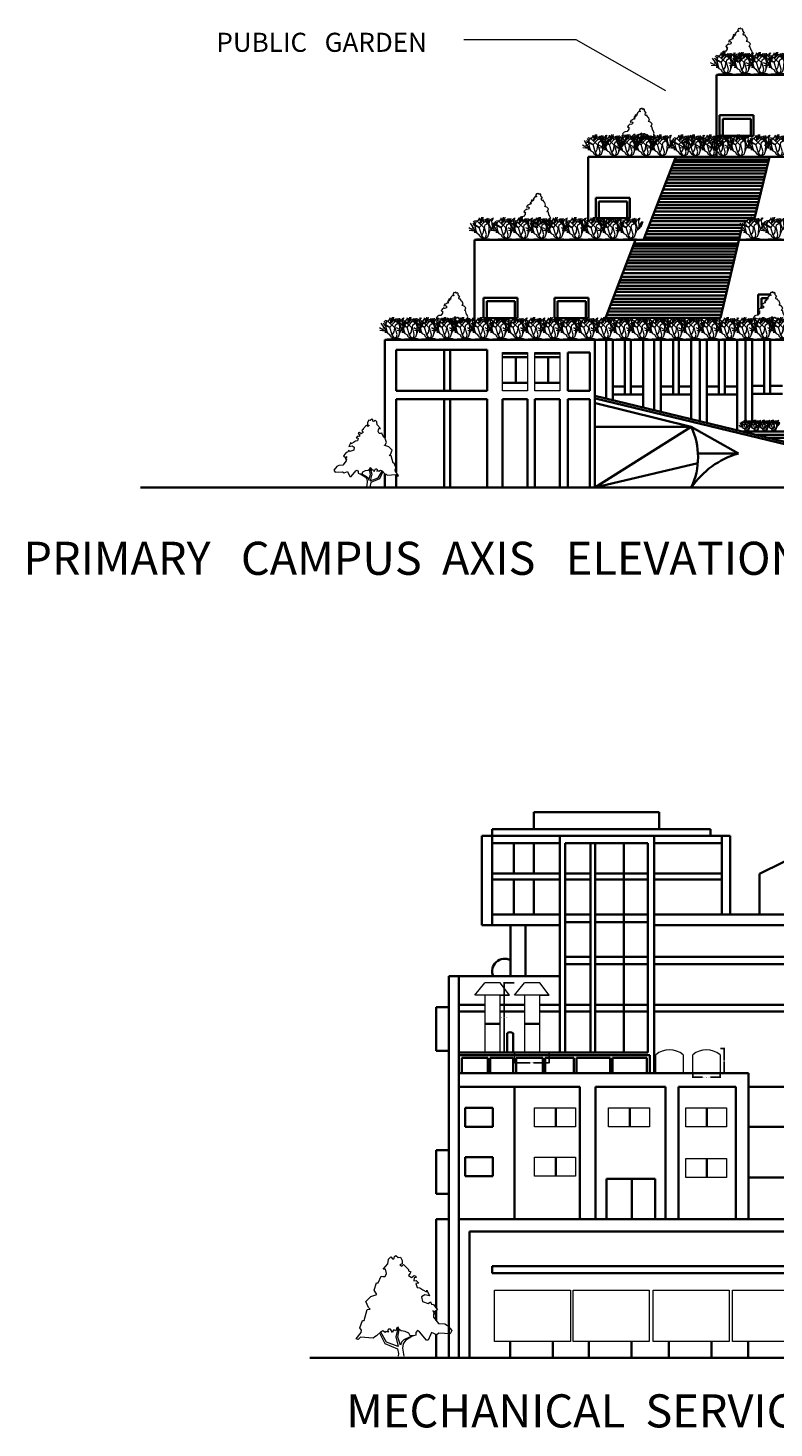
# Model space of a CAD drawing. Units: inches. Extents: x -362 to 223, y -437 to 70.
# Tile 1 of 5: x -362 to -124, y -437 to 8. Entities that reach past the tile are written whole.
import ezdxf

# ---------------------------------------------------------------- set-up
doc = ezdxf.new("R2010")
doc.units = ezdxf.units.IN
doc.header["$MEASUREMENT"] = 0
for name, color, linetype, lineweight in [('A-ANNO-DIMS', 2, 'Continuous', 18), ('A-ANNO-SYMB', 7, 'Continuous', 18), ('A-ANNO-TEXT', 7, 'Continuous', 25), ('A-ELEV', 7, 'Continuous', 35), ('A-EQPM', 8, 'Continuous', 18), ('A-GLAZ', 4, 'Continuous', 18), ('L-PLNT', 3, 'Continuous', 13)]:
    doc.layers.add(name, color=color, linetype=linetype, lineweight=lineweight)
doc.styles.get("Standard").update_dxf_attribs({"font": 'arial.ttf'})
doc.dimstyles.get("Standard").update_dxf_attribs({"dimtxt": 0.18, "dimasz": 0.18, "dimexe": 0.18, "dimexo": 0.0625, "dimgap": 0.09, "dimtad": 0, "dimtih": 1, "dimtoh": 1, "dimdec": 4, "dimzin": 0, "dimdsep": 46, "dimtxsty": 'Standard', "dimcen": 0.09, "dimadec": 0, "dimazin": 0, "dimtfac": 1, "dimtdec": 4, "dimtofl": 0, "dimtmove": 0, "dimatfit": 3, "dimfxl": 1, "dimtolj": 1, "dimtzin": 0, "dimarcsym": 0})

# ---------------------------------------------------------------- blocks, each defined once
blk = doc.blocks.new('*U2')
for points in [[(22.0124, 137.721), (18.5475, 141.5624), (15.5282, 138.2446), (13.8028, 139.3505), (13.3714, 142.1153), (11.2148, 143.2214), (8.1954, 140.4564), (4.7447, 141.0094), (2.1567, 136.0326), (2.1567, 131.6088), (5.6074, 129.9499), (3.0193, 128.2909), (0.4313, 130.5029), (-6.9015, 123.3141), (-6.9015, 121.6552), (-9.9208, 119.9963), (-9.0581, 118.3373), (-6.9015, 115.0195), (-10.7835, 112.2546), (-14.6656, 115.0195), (-16.8222, 114.4665), (-17.6849, 112.2546), (-14.6656, 111.7016), (-14.2342, 107.2778), (-17.6065, 107.8307), (-21.5669, 103.9599), (-17.2536, 103.4069), (-18.9789, 97.8771), (-22.8609, 97.3241), (-27.1743, 94.5593), (-32.3504, 91.7944), (-32.7817, 94.0063), (-36.6638, 85.7116), (-29.7624, 87.3705), (-25.449, 84.6056), (-26.743, 77.9699), (-34.507, 75.205), (-37.9578, 77.4169), (-39.2518, 74.099), (-42.2711, 73.5461), (-44.8592, 70.2282), (-47.8786, 66.3574), (-43.9965, 63.0395), (-41.4085, 64.6985), (-44.3346, 59.8898), (-42.2089, 60.1377), (-42.5159, 55.7849), (-49.6039, 46.4502), (-58.2307, 45.8972), (-62.1127, 43.6853), (-68.5828, 36.4966), (-65.9947, 32.0727), (-50.0352, 32.6257), (-47.0159, 30.4138), (-39.6831, 33.7317), (-34.507, 22.6721), (-32.3504, 22.6721), (-22.4296, 34.8376), (-19.4102, 36.4966), (-17.2536, 33.7317), (-17.2536, 29.8608), (-13.8028, 28.7549), (-9.0581, 28.7549), (-7.3328, 32.6257), (-1.7254, 35.3906), (3.8821, 35.9436), (6.4701, 38.1555), (6.9014, 38.7085), (8.1954, 41.4734), (9.9208, 40.3674), (11.2148, 35.9436), (14.2341, 37.6025), (15.0968, 36.4966), (15.9595, 33.7317), (18.9789, 38.7085), (21.9982, 38.7085), (23.2922, 36.4966), (21.9982, 34.2847), (25.4489, 35.3906), (26.743, 33.7317), (29.7623, 35.9436), (32.7817, 34.8376), (38.8204, 28.7549), (41.4084, 27.6489), (43.5651, 25.437), (61.6813, 27.0959), (65.132, 23.7781), (67.7201, 24.884), (60.8186, 33.7317), (60.3873, 37.0495), (62.544, 40.3674), (58.662, 50.874), (56.5053, 50.874), (52.1919, 66.3574), (47.8785, 66.9103), (50.4665, 69.1222), (53.9172, 77.9699), (47.0158, 85.1586), (38.3891, 87.9235), (42.2711, 94.0063)], [(42.2711, 94.0063), (38.8204, 104.5129), (36.6637, 104.5129), (32.3503, 113.9135), (29.7623, 113.3605), (26.743, 113.3605), (24.5862, 117.7844), (25.8802, 123.8671), (29.331, 123.8671), (22.8609, 131.6088), (21.9982, 137.6916)], [(8.1954, 40.3674), (11.2148, 27.6489), (8.1954, 13.8245), (24.5862, 19.9072), (32.7817, 34.2847)], [(-12.9401, 28.7549), (-2.588, 22.1191), (0.8626, 17.6953), (1.7253, 11.6125), (0, 0)], [(-9.9208, 28.2019), (0, 23.2251), (3.4507, 19.9072), (4.7447, 15.4834), (8.6267, 27.0959), (6.4701, 37.6025)], [(34.5071, 33.1787), (27.1743, 18.2483), (9.0581, 10.5066), (7.7641, 3.8708), (8.1954, 0)]]:
    blk.add_lwpolyline(points)
blk = doc.blocks.new('*U4')
for p, q in [((-18.24, 11.04), (-21.755, 16.655)), ((-12.96, 12.48), (-19.68, 16.32)), ((-13.92, 12.48), (-19.2, 14.88)), ((-16.8, 16.32), (-18.72, 18.72)), ((-14.88, 18.24), (-17.76, 19.2)), ((-16.8, 16.32), (-15.36, 19.68)), ((-16.8, 12.48), (-16.8, 16.32)), ((-14.88, 18.24), (-12.96, 20.64)), ((-8.16, 12), (-14.88, 18.24)), ((-13.325, 16.724), (-11.433, 18.289)), ((-12.96, 12.48), (-8.16, 17.76)), ((-12.471, 19.775), (-12.898, 22.044)), ((-11.677, 19.071), (-12.471, 19.775)), ((-11.28, 19.619), (-12.104, 21.184)), ((-12.043, 15.628), (-11.921, 18.836)), ((-11.982, 16.802), (-10.579, 18.054)), ((-11.921, 18.836), (-10.64, 20.401)), ((-11.433, 18.289), (-10.457, 22.749)), ((-10.579, 18.054), (-9.846, 19.697)), ((-8.16, 17.76), (-10.56, 21.6)), ((-9.48, 19.775), (-8.992, 22.592)), ((-7.2, 19.68), (-8.64, 20.16)), ((-8.16, 17.76), (-5.28, 19.2)), ((-7.68, 12.48), (-7.2, 14.88)), ((-7.2, 19.68), (-6.24, 21.12)), ((-4.8, 16.32), (-7.2, 19.68)), ((-7.2, 14.88), (-3.84, 16.8)), ((-5.086, 17.741), (-5.513, 21.34)), ((-5.28, 19.2), (-3.84, 21.6)), ((-3.377, 15.315), (-5.086, 17.819)), ((-2.88, 12.96), (-4.32, 19.68)), ((-3.84, 16.8), (-0.96, 20.64)), ((-3.377, 18.602), (-2.888, 21.575)), ((-2.766, 16.802), (-3.377, 18.602)), ((-2.88, 15.84), (-2.4, 20.16)), ((-0.96, 10.56), (-2.88, 15.84)), ((-0.508, 21.888), (-0.081, 20.558)), ((-0.203, 19.149), (0.102, 21.34)), ((0.346, 13.203), (-0.203, 19.149)), ((-0.142, 19.384), (0.59, 20.401)), ((-0.02, 20.01), (0.896, 21.105)), ((0.041, 20.714), (1.384, 22.044)), ((0.102, 21.34), (0.835, 21.888)), ((0.346, 13.203), (1.323, 16.254)), ((0.96, 12), (1.44, 15.36)), ((0.96, 12), (2.88, 14.88)), ((1.323, 16.254), (3.642, 18.289)), ((1.44, 15.36), (2.88, 17.28)), ((1.92, 13.44), (2.4, 15.36)), ((2.4, 15.36), (3.36, 16.32)), ((-17.76, 8.64), (-23.663, 11.961)), ((-17.76, 8.64), (-23.128, 9.222)), ((-18.24, 11.04), (-20.16, 11.52)), ((-15.84, 8.16), (-18.24, 11.04)), ((-16.32, 7.2), (-18.24, 7.2)), ((-16.8, 12.48), (-17.76, 12.96)), ((-14.88, 5.76), (-17.76, 8.64)), ((-15.84, 0.48), (-17.76, 0)), ((-15.84, 8.16), (-16.8, 12.48)), ((-14.88, 5.76), (-15.84, 8.16)), ((-13.44, 0.48), (-15.84, 0.48)), ((-12.96, 4.8), (-14.88, 5.76)), ((-12.96, 12.48), (-13.92, 12.48)), ((-9.6, 0.96), (-13.44, 0.48)), ((-10.56, 4.32), (-12.96, 12.48)), ((-11.52, 2.4), (-12.96, 4.8)), ((-9.6, 0.96), (-12.96, 0)), ((-8.64, 0.96), (-11.52, 2.4)), ((-10.56, 4.32), (-8.64, 7.68)), ((-8.64, 1.92), (-10.56, 4.32)), ((-9.6, 0.96), (-7.68, 0.96)), ((-8.64, 7.68), (-8.16, 12)), ((-8.64, 0.96), (-4.32, 2.88)), ((-8.64, 0.96), (-6.24, 2.88)), ((-8.64, 0.96), (-8.64, 1.92)), ((-8.64, 0.96), (-2.88, 0.96)), ((-6.72, 8.64), (-7.68, 12.48)), ((-7.68, 0.96), (-6.24, 0.48)), ((-5.76, 5.28), (-6.72, 8.64)), ((-6.24, 2.88), (-5.76, 5.28)), ((-6.24, 0.48), (-3.36, 0)), ((-4.32, 2.88), (-1.92, 9.6)), ((-3.36, 5.28), (-2.88, 12.96)), ((-2.88, 0.96), (0, 0)), ((-1.92, 9.6), (0.96, 12)), ((-0.48, 10.8), (0.346, 13.203))]:
    blk.add_line(p, q)
blk = doc.blocks.new('WIN-PANEL-A')
for p, q in [((0, 12.16), (7.9, 12.16)), ((0, 0), (0, 12.16)), ((7.9, 12.16), (7.9, 0)), ((7.9, 0), (0, 0))]:
    blk.add_line(p, q)
blk = doc.blocks.new('WIN-STOREFRONT')
for p, q in [((24.23, 16.39), (0, 16.39)), ((0, 16.39), (0, 0)), ((24.23, 0), (24.23, 16.39)), ((0, 0), (6.79, 0)), ((6.79, 0), (24.23, 0))]:
    blk.add_line(p, q)
blk = doc.blocks.new('ROOF-VENT')
for p, q in [((0, 18.24), (2.99, 22.1)), ((2.99, 18.24), (0, 18.24)), ((0, 18.24), (11.03, 18.24)), ((2.99, 22.1), (7.83, 22.1)), ((2.99, 0), (2.99, 18.24)), ((2.99, 18.24), (7.83, 18.24)), ((11.03, 18.24), (7.83, 22.1)), ((7.83, 18.24), (7.83, 0))]:
    blk.add_line(p, q)
blk = doc.blocks.new('WIN-C')
for p, q in [((13.02, 6.07), (0, 6.07)), ((0, 6.07), (0, 5.53)), ((0, 5.53), (0, 0)), ((13.02, 0), (13.02, 6.07)), ((0, 0), (13.02, 0))]:
    blk.add_line(p, q)
blk = doc.blocks.new('WIN-D')
for p, q in [((13.02, 6.07), (0, 6.07)), ((0, 6.07), (0, 5.53)), ((0, 5.53), (0, 0)), ((13.02, 6.07), (11.9, 6.07)), ((13.02, 0), (13.02, 6.07)), ((0, 0), (13.02, 0)), ((11.9, 0), (13.02, 0))]:
    blk.add_line(p, q)
blk = doc.blocks.new('ROOF-DOME')
for p, q in [((0, 0), (0, 5.87)), ((8.74, 5.87), (8.74, 0))]:
    blk.add_line(p, q)
blk.add_arc((4.37, 0.37), 7.03, 51.5309, 128.4691)
blk = doc.blocks.new('*D27')
at = {"layer": 'A-ANNO-DIMS', "color": 0, "lineweight": -2, "transparency": 16777216}
for p, q in [((-207, -295.53), (-210.43, -295.53)), ((-210.25, -295.71), (-210.25, -306.39)), ((-210.25, -317.45), (-210.25, -306.76)), ((-207, -317.63), (-210.43, -317.63))]:
    blk.add_line(p, q, dxfattribs=at)
at = {"layer": 'A-ANNO-DIMS', "color": 0, "transparency": 16777216}
for points in [[(-210.28, -295.71), (-210.22, -295.71), (-210.25, -295.53)], [(-210.28, -317.45), (-210.22, -317.45), (-210.25, -317.63)]]:
    blk.add_solid(points, dxfattribs=at)
at = {"layer": 'Defpoints', "color": 0, "transparency": 16777216}
for p in [(-210.25, -295.53), (-206.94, -295.53), (-206.94, -317.63)]:
    blk.add_point(p, dxfattribs=at)
at = {"layer": 'A-ANNO-DIMS', "color": 0, "transparency": 16777216, "insert": (-210.25, -306.58), "char_height": 0.18, "attachment_point": 5}
blk.add_mtext('\\A1;ROOF VENT 22 TYP.', dxfattribs=at)
blk = doc.blocks.new('*D28')
at = {"layer": 'A-ANNO-DIMS', "color": 0, "lineweight": -2, "transparency": 16777216}
for p, q in [((-206.94, -317.69), (-206.94, -321.12)), ((-195.91, -317.69), (-195.91, -321.12)), ((-206.76, -320.94), (-201.94, -320.94)), ((-196.09, -320.94), (-200.9, -320.94))]:
    blk.add_line(p, q, dxfattribs=at)
at = {"layer": 'A-ANNO-DIMS', "color": 0, "transparency": 16777216}
for points in [[(-206.76, -320.91), (-206.76, -320.97), (-206.94, -320.94)], [(-196.09, -320.91), (-196.09, -320.97), (-195.91, -320.94)]]:
    blk.add_solid(points, dxfattribs=at)
at = {"layer": 'Defpoints', "color": 0, "transparency": 16777216}
for p in [(-206.94, -317.63), (-195.91, -317.63), (-206.94, -320.94)]:
    blk.add_point(p, dxfattribs=at)
at = {"layer": 'A-ANNO-DIMS', "color": 0, "transparency": 16777216, "insert": (-201.42, -320.94), "char_height": 0.18, "attachment_point": 5}
blk.add_mtext('\\A1;11 TYP.', dxfattribs=at)
blk = doc.blocks.new('*D31')
at = {"layer": 'A-ANNO-DIMS', "color": 0, "lineweight": -2, "transparency": 16777216}
for p, q in [((-150.17, -324.32), (-150.17, -325.75)), ((-141.42, -324.32), (-141.42, -325.75)), ((-149.99, -325.57), (-147.06, -325.57)), ((-141.6, -325.57), (-144.53, -325.57))]:
    blk.add_line(p, q, dxfattribs=at)
at = {"layer": 'A-ANNO-DIMS', "color": 0, "transparency": 16777216}
for points in [[(-149.99, -325.54), (-149.99, -325.6), (-150.17, -325.57)], [(-141.6, -325.54), (-141.6, -325.6), (-141.42, -325.57)]]:
    blk.add_solid(points, dxfattribs=at)
at = {"layer": 'Defpoints', "color": 0, "transparency": 16777216}
for p in [(-150.17, -324.26), (-141.42, -324.26), (-141.42, -325.57)]:
    blk.add_point(p, dxfattribs=at)
at = {"layer": 'A-ANNO-DIMS', "color": 0, "transparency": 16777216, "insert": (-145.8, -325.57), "char_height": 0.18, "attachment_point": 5}
blk.add_mtext('\\A1;ROOF DOME 9 TYP.', dxfattribs=at)
blk = doc.blocks.new('*D32')
at = {"layer": 'A-ANNO-DIMS', "color": 0, "lineweight": -2, "transparency": 16777216}
for p, q in [((-141.36, -316.35), (-139.93, -316.35)), ((-140.11, -316.53), (-140.11, -320.12)), ((-140.11, -324.08), (-140.11, -320.49)), ((-141.36, -324.26), (-139.93, -324.26))]:
    blk.add_line(p, q, dxfattribs=at)
at = {"layer": 'A-ANNO-DIMS', "color": 0, "transparency": 16777216}
for points in [[(-140.14, -316.53), (-140.08, -316.53), (-140.11, -316.35)], [(-140.14, -324.08), (-140.08, -324.08), (-140.11, -324.26)]]:
    blk.add_solid(points, dxfattribs=at)
at = {"layer": 'Defpoints', "color": 0, "transparency": 16777216}
for p in [(-141.42, -316.35), (-140.11, -316.35), (-141.42, -324.26)]:
    blk.add_point(p, dxfattribs=at)
at = {"layer": 'A-ANNO-DIMS', "color": 0, "transparency": 16777216, "insert": (-140.11, -320.3), "char_height": 0.18, "attachment_point": 5}
blk.add_mtext('\\A1;8 TYP.', dxfattribs=at)

msp = doc.modelspace()

# ---------------------------------------------------------------- linework, layer by layer
at = {"layer": 'A-ANNO-SYMB'}
for p, q in [((-187.3, 4.66), (-223.08, 4.66)), ((-158.77, -11.54), (-187.3, 4.66))]:
    msp.add_line(p, q, dxfattribs=at)
at = {"layer": 'A-ELEV'}
for p, q in [((-62.22, -6.5), (-142.63, -6.5)), ((-142.63, -6.5), (-142.63, -25.83)), ((-141.63, -25.83), (-141.63, -19.35)), ((-141.63, -19.35), (-130.81, -19.35)), ((-140.6, -20.44), (-131.66, -20.44)), ((-140.6, -25.83), (-140.6, -20.44)), ((-131.66, -25.83), (-131.66, -20.44)), ((-130.81, -19.35), (-130.81, -25.83)), ((-142.63, -25.83), (-142.63, -32.58)), ((-141.63, -25.83), (-130.81, -25.83)), ((-183.41, -32.58), (-183.41, -53.27)), ((-80.64, -32.58), (-183.41, -32.58)), ((-165.87, -59), (-155.5, -32.58)), ((-156.5, -35.12), (-126.36, -35.12)), ((-156.13, -34.18), (-126.14, -34.18)), ((-155.83, -33.43), (-125.96, -33.43)), ((-155.5, -32.58), (-125.62, -32.58)), ((-130.35, -51.77), (-125.75, -32.58)), ((-158.31, -39.74), (-127.47, -39.74)), ((-157.99, -38.93), (-127.27, -38.93)), ((-157.58, -37.87), (-127.02, -37.87)), ((-157.21, -36.93), (-126.79, -36.93)), ((-156.86, -36.05), (-126.58, -36.05)), ((-160.03, -44.13), (-128.52, -44.13)), ((-159.57, -42.94), (-128.23, -42.94)), ((-159.12, -41.8), (-127.96, -41.8)), ((-158.73, -40.8), (-127.72, -40.8)), ((-181.05, -52.14), (-181.05, -45.65)), ((-181.05, -45.65), (-170.24, -45.65)), ((-180.03, -46.74), (-171.09, -46.74)), ((-180.03, -52.13), (-180.03, -46.74)), ((-171.09, -52.13), (-171.09, -46.74)), ((-170.24, -45.65), (-170.24, -52.13)), ((-161.9, -48.88), (-129.65, -48.88)), ((-161.53, -47.94), (-129.43, -47.94)), ((-161.16, -47), (-129.21, -47)), ((-160.75, -45.94), (-128.95, -45.94)), ((-160.4, -45.07), (-128.74, -45.07)), ((-181.05, -52.13), (-170.24, -52.13)), ((-166.17, -53.17), (-166.81, -54.85)), ((-163.53, -53.03), (-132.81, -53.03)), ((-162.76, -51.08), (-130.18, -51.08)), ((-162.76, -52.08), (-130.18, -52.08)), ((-162.34, -50.01), (-129.92, -50.01)), ((-131.96, -53.03), (-131.46, -53.03)), ((-126.36, -53.03), (-125.96, -53.03)), ((-183.41, -54.5), (-183.41, -54.74)), ((-183.41, -56.44), (-183.41, -56.85)), ((-165.15, -57.16), (-134.98, -57.16)), ((-164.78, -56.22), (-134.76, -56.22)), ((-164.36, -55.16), (-134.49, -55.16)), ((-164, -54.22), (-133.49, -54.22)), ((-134.72, -56.05), (-141.34, -83.84)), ((-134.51, -55.17), (-134.53, -55.25)), ((-134.49, -55.16), (-134.51, -55.17)), ((-132.98, -54.22), (-133.04, -54.26)), ((-219.64, -59), (-92.76, -59)), ((-183.41, -59), (-219.64, -59)), ((-219.64, -59), (-219.64, -84.82)), ((-183.41, -58.78), (-183.41, -59)), ((-168.38, -58.94), (-178.17, -84.48)), ((-169.34, -61.79), (-136.09, -61.79)), ((-168.97, -60.85), (-135.86, -60.85)), ((-168.68, -60.1), (-135.68, -60.1)), ((-165.57, -58.22), (-135.24, -58.22)), ((-171.16, -66.41), (-137.19, -66.41)), ((-170.84, -65.6), (-136.99, -65.6)), ((-170.42, -64.54), (-136.74, -64.54)), ((-170.05, -63.6), (-136.52, -63.6)), ((-169.71, -62.72), (-136.31, -62.72)), ((-172.88, -70.8), (-138.23, -70.8)), ((-172.41, -69.61), (-137.95, -69.61)), ((-171.97, -68.47), (-137.68, -68.47)), ((-171.57, -67.47), (-137.44, -67.47)), ((-174.74, -75.55), (-139.36, -75.55)), ((-174.38, -74.61), (-139.14, -74.61)), ((-174.01, -73.67), (-138.92, -73.67)), ((-173.59, -72.61), (-138.66, -72.61)), ((-173.25, -71.74), (-138.46, -71.74)), ((-216.78, -83.93), (-216.78, -77.44)), ((-216.78, -77.44), (-205.97, -77.44)), ((-215.76, -78.53), (-206.82, -78.53)), ((-215.76, -83.92), (-215.76, -78.53)), ((-206.82, -83.92), (-206.82, -78.53)), ((-205.97, -77.44), (-205.97, -83.92)), ((-194.19, -83.93), (-194.19, -77.44)), ((-194.19, -77.44), (-183.38, -77.44)), ((-193.17, -78.53), (-184.23, -78.53)), ((-193.17, -83.92), (-193.17, -78.53)), ((-184.23, -83.92), (-184.23, -78.53)), ((-183.38, -77.44), (-183.38, -83.92)), ((-176.37, -79.7), (-140.35, -79.7)), ((-175.61, -77.75), (-139.89, -77.75)), ((-175.61, -78.75), (-140.13, -78.75)), ((-175.18, -76.68), (-139.63, -76.68)), ((-129.33, -82.9), (-129.33, -76.41)), ((-129.33, -76.41), (-125.46, -76.41)), ((-128.3, -77.5), (-126.3, -77.5)), ((-128.3, -79.69), (-128.3, -77.5)), ((-128.3, -80.78), (-128.3, -79.96)), ((-216.78, -83.92), (-205.97, -83.92)), ((-194.19, -83.92), (-183.38, -83.92)), ((-177.99, -83.83), (-141.34, -83.83)), ((-177.62, -82.89), (-141.11, -82.89)), ((-177.21, -81.83), (-140.86, -81.83)), ((-176.84, -80.89), (-140.64, -80.89)), ((-219.64, -85.32), (-219.64, -85.5)), ((-219.64, -86.44), (-219.64, -86.6)), ((-219.64, -88.43), (-219.64, -88.46)), ((-248.18, -90.83), (-105.32, -90.83)), ((-248.18, -90.83), (-248.18, -121.99)), ((-194.27, -90.83), (-188.3, -90.83)), ((-181.3, -90.83), (-181.3, -137.85)), ((-177.76, -90.83), (-177.76, -109.45)), ((-175.62, -90.83), (-175.62, -108.18)), ((-171.74, -108.18), (-171.74, -90.83)), ((-169.85, -90.83), (-169.85, -108.18)), ((-165.97, -108.18), (-165.97, -90.83)), ((-162.45, -90.83), (-162.45, -113.16)), ((-160.31, -90.83), (-160.31, -108.18)), ((-156.43, -108.18), (-156.43, -90.83)), ((-154.54, -90.83), (-154.54, -108.18)), ((-150.66, -108.18), (-150.66, -90.83)), ((-147.85, -90.83), (-147.85, -116.71)), ((-145.71, -90.83), (-145.71, -108.18)), ((-141.83, -108.18), (-141.83, -90.83)), ((-139.94, -90.83), (-139.94, -108.18)), ((-136.06, -108.18), (-136.06, -90.83)), ((-133.39, -90.65), (-133.39, -116.8)), ((-131.26, -90.65), (-131.26, -108)), ((-127.38, -108), (-127.38, -90.65)), ((-125.49, -90.65), (-125.49, -108)), ((-244.61, -94.01), (-244.61, -107.01)), ((-215.61, -94.01), (-244.61, -94.01)), ((-229.33, -94.01), (-229.33, -107.01)), ((-229.33, -94.01), (-229.33, -107.01)), ((-227.35, -94.01), (-227.35, -107.01)), ((-215.61, -107.01), (-215.61, -94.01)), ((-210.69, -95.2), (-202.79, -95.2)), ((-210.69, -96.36), (-202.79, -96.36)), ((-206.49, -104.5), (-206.49, -96.36)), ((-200.43, -95.2), (-192.52, -95.2)), ((-200.43, -96.36), (-192.52, -96.36)), ((-196.22, -104.5), (-196.22, -96.36)), ((-189.95, -94.88), (-189.95, -107.04)), ((-182.89, -94.88), (-189.95, -94.88)), ((-182.89, -107.04), (-182.89, -94.88)), ((-210.69, -104.5), (-202.79, -104.5)), ((-200.43, -104.5), (-192.52, -104.5)), ((-175.62, -105.68), (-171.74, -105.68)), ((-169.85, -105.68), (-165.97, -105.68)), ((-160.31, -105.68), (-156.43, -105.68)), ((-154.54, -105.68), (-150.66, -105.68)), ((-145.71, -105.68), (-141.83, -105.68)), ((-139.94, -105.68), (-136.06, -105.68)), ((-131.26, -105.5), (-127.38, -105.5)), ((-125.49, -105.5), (-121.61, -105.5)), ((-244.61, -107.01), (-215.61, -107.01)), ((-244.61, -109.74), (-244.61, -132.99)), ((-244.61, -109.74), (-215.61, -109.74)), ((-229.33, -109.74), (-229.33, -137.85)), ((-229.33, -109.74), (-229.33, -137.85)), ((-227.35, -109.74), (-227.35, -137.85)), ((-215.61, -109.74), (-215.61, -137.85)), ((-210.69, -109.74), (-210.69, -137.85)), ((-210.69, -109.74), (-202.79, -109.74)), ((-202.79, -109.74), (-202.79, -137.85)), ((-200.43, -109.74), (-200.43, -137.85)), ((-200.43, -109.74), (-192.52, -109.74)), ((-192.52, -109.74), (-192.52, -137.85)), ((-189.95, -107.04), (-182.89, -107.04)), ((-189.95, -109.74), (-189.95, -137.85)), ((-189.95, -109.74), (-182.89, -109.74)), ((-182.89, -109.74), (-182.89, -137.85)), ((-181.3, -108.59), (-60.7, -137.85)), ((-181.11, -109.51), (-63.64, -137.85)), ((-181.11, -111.01), (-150.61, -118.51)), ((-175.62, -108.18), (-171.74, -108.18)), ((-175.62, -108.18), (-165.97, -108.18)), ((-175.62, -108.18), (-175.62, -109.97)), ((-169.85, -108.18), (-165.97, -108.18)), ((-165.97, -108.18), (-165.97, -112.31)), ((-160.31, -108.18), (-156.43, -108.18)), ((-160.31, -108.18), (-150.66, -108.18)), ((-160.31, -108.18), (-160.31, -113.68)), ((-154.54, -108.18), (-150.66, -108.18)), ((-150.66, -108.18), (-150.66, -116.02)), ((-145.71, -108.18), (-141.83, -108.18)), ((-145.71, -108.18), (-136.06, -108.18)), ((-145.71, -108.18), (-145.71, -117.23)), ((-139.94, -108.18), (-136.06, -108.18)), ((-136.06, -108.18), (-136.06, -119.57)), ((-131.26, -108), (-127.38, -108)), ((-131.26, -108), (-121.61, -108)), ((-131.26, -108), (-131.26, -116.68)), ((-125.49, -108), (-121.61, -108)), ((-150.61, -118.51), (-181.3, -118.51)), ((-150.61, -118.51), (-181.3, -137.85)), ((-150.61, -118.51), (-135.58, -127.01)), ((-61.89, -120.01), (-134.22, -120.01)), ((-248.18, -124.35), (-248.18, -124.49)), ((-130.1, -121.01), (-55.47, -121.01)), ((-125.98, -122.01), (-55.34, -122.01)), ((-135.58, -127.01), (-148.51, -127.01)), ((-248.18, -133.44), (-248.18, -137.85)), ((-181.3, -137.85), (-148.56, -130.09)), ((-248.18, -137.85), (-326.06, -137.85)), ((-248.18, -137.85), (-188.3, -137.85)), ((-244.61, -133.79), (-244.61, -137.85)), ((-188.3, -137.85), (-28, -137.85)), ((-160.86, -241.22), (-200.81, -241.22)), ((-200.81, -241.22), (-200.81, -246.58)), ((-160.86, -246.58), (-160.86, -241.22)), ((-213.99, -248.69), (-217.3, -248.69)), ((-217.3, -248.69), (-217.3, -273.74)), ((-213.99, -277.1), (-213.99, -246.58)), ((-213.99, -246.58), (-144.55, -246.58)), ((-144.55, -248.69), (-213.99, -248.69)), ((-192.44, -248.69), (-192.44, -317.63)), ((-162.48, -248.72), (-162.48, -317.63)), ((-144.55, -246.58), (-144.55, -248.69)), ((-144.55, -248.69), (-138.19, -248.69)), ((-140.92, -273.74), (-140.92, -248.69)), ((-138.19, -248.69), (-138.19, -273.74)), ((-128.95, -260.83), (-105.16, -249.03)), ((-192.44, -251.06), (-213.99, -251.06)), ((-207.18, -251.06), (-207.18, -260.65)), ((-200.81, -251.06), (-200.81, -260.65)), ((-165.03, -251.06), (-190.73, -251.06)), ((-190.73, -251.06), (-190.73, -317.63)), ((-182.71, -251.06), (-190.73, -251.06)), ((-182.71, -251.06), (-182.71, -317.63)), ((-181.24, -251.06), (-181.24, -317.63)), ((-164.44, -251.06), (-181.24, -251.06)), ((-172.13, -251.06), (-172.13, -317.63)), ((-165.03, -251.06), (-164.44, -251.06)), ((-164.44, -251.06), (-164.44, -317.63)), ((-140.92, -251.06), (-162.48, -251.06)), ((-192.44, -260.65), (-213.99, -260.65)), ((-192.44, -262.59), (-213.99, -262.59)), ((-207.18, -262.59), (-207.18, -273.74)), ((-200.81, -262.59), (-200.81, -273.74)), ((-182.71, -260.65), (-190.73, -260.65)), ((-182.71, -262.59), (-190.73, -262.59)), ((-164.44, -260.65), (-181.24, -260.65)), ((-164.44, -262.59), (-181.24, -262.59)), ((-140.92, -260.65), (-162.48, -260.65)), ((-140.92, -262.59), (-162.48, -262.59)), ((-128.95, -273.74), (-128.95, -260.83)), ((-217.3, -273.74), (-217.3, -277.1)), ((-192.44, -273.74), (-213.99, -273.74)), ((-182.71, -273.74), (-190.73, -273.74)), ((-182.71, -276.18), (-190.73, -276.18)), ((-164.44, -273.74), (-181.24, -273.74)), ((-164.44, -276.18), (-181.24, -276.18)), ((-140.92, -273.74), (-162.48, -273.74)), ((-138.19, -273.74), (-140.92, -273.74)), ((-138.19, -273.74), (-97.81, -273.74)), ((-217.3, -277.1), (-213.99, -277.1)), ((-192.44, -277.1), (-213.99, -277.1)), ((-213.99, -277.1), (-192.44, -277.1)), ((-208.15, -277.1), (-208.15, -288.32)), ((-203.39, -277.1), (-203.39, -288.32)), ((-140.92, -277.1), (-162.48, -277.1)), ((-162.48, -277.1), (-105.45, -277.1)), ((-208.15, -288.32), (-208.15, -293.39)), ((-203.39, -288.32), (-203.39, -293.39)), ((-182.71, -287.17), (-190.73, -287.17)), ((-182.71, -289.53), (-190.73, -289.53)), ((-164.44, -287.17), (-181.24, -287.17)), ((-164.44, -289.53), (-181.24, -289.53)), ((-162.48, -289.53), (-75.93, -289.53)), ((-224.68, -293.39), (-227.83, -293.39)), ((-227.83, -293.39), (-227.83, -370.73)), ((-203.39, -293.39), (-224.68, -293.39)), ((-224.68, -293.39), (-224.68, -338.07)), ((-203.39, -293.39), (-192.44, -293.39)), ((-216.36, -302.45), (-224.68, -302.45)), ((-203.74, -302.45), (-211.52, -302.45)), ((-192.44, -302.45), (-198.9, -302.45)), ((-182.71, -302.45), (-190.73, -302.45)), ((-164.44, -302.45), (-181.24, -302.45)), ((-162.48, -302.45), (-75.93, -302.45)), ((-227.83, -303.22), (-231.85, -303.22)), ((-231.85, -303.22), (-231.85, -313.58)), ((-216.36, -304.65), (-224.68, -304.65)), ((-203.74, -304.65), (-211.52, -304.65)), ((-192.44, -304.65), (-198.9, -304.65)), ((-182.71, -304.65), (-190.73, -304.65)), ((-164.44, -304.65), (-181.24, -304.65)), ((-162.48, -304.65), (-75.93, -304.65)), ((-211.52, -308.56), (-216.36, -308.56)), ((-209.22, -311.48), (-209.22, -317.63)), ((-207.38, -317.63), (-207.38, -311.48)), ((-207.38, -311.48), (-207.38, -311.48)), ((-198.9, -308.56), (-203.74, -308.56)), ((-231.85, -313.58), (-231.85, -317.17)), ((-231.85, -317.17), (-227.83, -317.17)), ((-224.68, -317.63), (-164.44, -317.63)), ((-163.81, -318.52), (-224.68, -318.52)), ((-215.43, -319.37), (-223.67, -319.37)), ((-223.67, -324.26), (-223.67, -319.37)), ((-215.43, -324.26), (-215.43, -319.37)), ((-207.3, -319.37), (-214.65, -319.37)), ((-214.65, -324.26), (-214.65, -319.37)), ((-207.3, -324.26), (-207.3, -319.37)), ((-197.9, -319.37), (-206.41, -319.37)), ((-206.41, -324.26), (-206.41, -319.37)), ((-197.9, -324.26), (-197.9, -319.37)), ((-187.99, -319.37), (-197.12, -319.37)), ((-197.12, -324.26), (-197.12, -319.37)), ((-187.99, -324.26), (-187.99, -319.37)), ((-176.47, -319.37), (-187.21, -319.37)), ((-187.21, -324.26), (-187.21, -319.37)), ((-176.47, -324.26), (-176.47, -319.37)), ((-164.8, -319.37), (-175.74, -319.37)), ((-175.74, -324.26), (-175.74, -319.37)), ((-164.8, -324.26), (-164.8, -319.37)), ((-163.83, -324.26), (-163.83, -319.37)), ((-163.81, -319.37), (-163.81, -318.52)), ((-162.48, -317.63), (-162.48, -324.26)), ((-132.36, -324.26), (-224.68, -324.26)), ((-132.36, -370.73), (-132.36, -324.26)), ((-186.07, -328.62), (-224.68, -328.62)), ((-206.95, -328.62), (-206.95, -370.73)), ((-186.07, -328.62), (-186.07, -370.73)), ((-158.87, -328.62), (-181.12, -328.62)), ((-181.12, -328.62), (-181.12, -370.73)), ((-158.87, -328.62), (-158.87, -370.73)), ((-136.46, -328.62), (-154.74, -328.62)), ((-154.74, -328.62), (-154.74, -370.73)), ((-136.46, -370.73), (-136.46, -328.62)), ((-132.36, -328.62), (-75.93, -328.62)), ((-224.68, -338.07), (-224.68, -370.73)), ((-222.58, -341.31), (-222.58, -335.24)), ((-222.58, -335.24), (-213.85, -335.24)), ((-213.85, -335.24), (-213.85, -341.31)), ((-193.75, -335.24), (-193.75, -341.31)), ((-170.16, -335.24), (-170.16, -341.31)), ((-145.62, -335.24), (-145.62, -341.31)), ((-213.85, -341.31), (-222.58, -341.31)), ((-132.36, -341.31), (-95.58, -341.31)), ((-227.83, -348.77), (-231.85, -348.77)), ((-231.85, -348.77), (-231.85, -359.13)), ((-222.58, -357.09), (-222.58, -351.02)), ((-222.58, -351.02), (-213.85, -351.02)), ((-213.85, -351.02), (-213.85, -357.09)), ((-193.75, -351.02), (-193.75, -357.09)), ((-145.62, -351.45), (-145.62, -357.51)), ((-231.85, -359.13), (-231.85, -362.71)), ((-213.85, -357.09), (-222.58, -357.09)), ((-162.16, -357.88), (-177.59, -357.88)), ((-177.59, -357.88), (-177.59, -370.73)), ((-169.53, -370.73), (-169.53, -357.88)), ((-162.16, -370.73), (-162.16, -357.88)), ((-132.36, -357.51), (-85.99, -357.51)), ((-231.85, -362.71), (-227.83, -362.71)), ((-227.83, -370.73), (-231.84, -370.73)), ((-231.84, -370.73), (-231.84, -399.03)), ((-227.83, -370.73), (-227.83, -414.88)), ((-224.68, -370.73), (-85.99, -370.73)), ((-224.68, -370.73), (-224.68, -414.88)), ((-221.28, -414.88), (-221.28, -374.68)), ((-221.28, -374.68), (-85.99, -374.68)), ((-85.99, -385.66), (-214.01, -385.66)), ((-214.01, -385.66), (-214.01, -387.9)), ((-85.99, -387.9), (-214.01, -387.9)), ((-231.84, -399.84), (-231.84, -402.96)), ((-231.84, -407.47), (-231.84, -414.88)), ((-208.31, -414.77), (-208.31, -409.69)), ((-194.72, -414.77), (-194.72, -409.69)), ((-183.24, -414.77), (-183.24, -409.69)), ((-169.65, -414.77), (-169.65, -409.69)), ((-157.74, -414.77), (-157.74, -409.69)), ((-144.15, -414.77), (-144.15, -409.69)), ((-132.53, -414.77), (-132.53, -409.69)), ((-227.83, -414.88), (-272.1, -414.88)), ((-231.84, -414.88), (-224.68, -414.88)), ((-224.68, -414.88), (-75.93, -414.88)), ((-25.37, -414.88), (-130.92, -414.88))]:
    msp.add_line(p, q, dxfattribs=at)
msp.add_lwpolyline([(-162.48, -287.17), (-75.93, -287.17)], dxfattribs=at)
for centre, radius, start, end in [((-171.48, -128.18), 23, 335.1387, 24.8613), ((-128.06, -153.27), 27.32, 105.9751, 145.6417), ((-210.05, -291.82), 3.98, 61.4732, 203.1687), ((-208.3, -312.87), 1.66, 56.4994, 123.5006)]:
    msp.add_arc(centre, radius, start, end, dxfattribs=at)

# ---------------------------------------------------------------- block references
at = {"layer": 'A-EQPM', "extrusion": (0, 0, -1), "zscale": -1}
for p in [(208.53, -317.63), (195.91, -317.63)]:
    msp.add_blockref('ROOF-VENT', p, dxfattribs=at)
at = {"layer": 'A-EQPM'}
for p in [(-161.94, -324.25), (-150.17, -324.25)]:
    msp.add_blockref('ROOF-DOME', p, dxfattribs=at)
at = {"layer": 'A-GLAZ', "rotation": 180}
for p in [(-202.79, -94.88), (-192.52, -94.88)]:
    msp.add_blockref('WIN-PANEL-A', p, dxfattribs=at)
at = {"layer": 'A-GLAZ', "extrusion": (0, 0, -1), "zscale": -1}
for name, p in [('WIN-D', (187.5, -341.31)), ('WIN-C', (163.91, -341.31)), ('WIN-C', (139.38, -341.31)), ('WIN-D', (187.5, -357.09)), ('WIN-C', (139.38, -357.51)), ('WIN-STOREFRONT', (189.08, -409.69)), ('WIN-STOREFRONT', (164.01, -409.69)), ('WIN-STOREFRONT', (138.51, -409.69)), ('WIN-STOREFRONT', (113.3, -409.69))]:
    msp.add_blockref(name, p, dxfattribs=at)
at = {"layer": 'L-PLNT'}
for name, p, xscale, yscale, zscale in [('*U2', (-135.95, -2.57), 0.0769249465327344, 0.0769249465327344, 0.0769249465327344), ('*U4', (-137, -6.36), 0.3151431067188808, 0.3151431067188808, 0.3151431067188808), ('*U4', (-131.2, -6.36), 0.3151431067188808, 0.3151431067188808, 0.3151431067188808), ('*U4', (-125.74, -6.36), 0.3151431067188808, 0.3151431067188808, 0.3151431067188808), ('*U4', (-120.18, -6.36), 0.3151431067188808, 0.3151431067188808, 0.3151431067188808), ('*U2', (-167.23, -28.09), 0.0769249465327344, 0.0769249465327344, 0.0769249465327344), ('*U4', (-177.82, -32.6), 0.3151431067188808, 0.3151431067188808, 0.3151431067188808), ('*U4', (-172.6, -32.6), 0.3151431067188808, 0.3151431067188808, 0.3151431067188808), ('*U4', (-167.68, -32.6), 0.3151431067188808, 0.3151431067188808, 0.3151431067188808), ('*U4', (-162.51, -32.6), 0.3151431067188808, 0.3151431067188808, 0.3151431067188808), ('*U4', (-157.33, -32.6), 0.3151431067188808, 0.3151431067188808, 0.3151431067188808), ('*U4', (-150.47, -32.6), 0.3151431067188808, 0.3151431067188808, 0.3151431067188808), ('*U4', (-146.76, -32.6), 0.3151431067188808, 0.3151431067188808, 0.3151431067188808), ('*U4', (-141.46, -32.6), 0.3151431067188808, 0.3151431067188808, 0.3151431067188808), ('*U4', (-137.98, -32.6), 0.3151431067188808, 0.3151431067188808, 0.3151431067188808), ('*U4', (-132.45, -32.6), 0.3151431067188808, 0.3151431067188808, 0.3151431067188808), ('*U4', (-125.94, -32.6), 0.3151431067188808, 0.3151431067188808, 0.3151431067188808), ('*U4', (-119.81, -32.6), 0.3151431067188808, 0.3151431067188808, 0.3151431067188808), ('*U2', (-200.26, -55.16), 0.0769249465327344, 0.0769249465327344, 0.0769249465327344), ('*U4', (-214.03, -58.94), 0.3151431067188808, 0.3151431067188808, 0.3151431067188808), ('*U4', (-207.09, -58.94), 0.3151431067188808, 0.3151431067188808, 0.3151431067188808), ('*U4', (-201.52, -58.94), 0.3151431067188808, 0.3151431067188808, 0.3151431067188808), ('*U4', (-195.81, -58.94), 0.3151431067188808, 0.3151431067188808, 0.3151431067188808), ('*U4', (-190.43, -58.94), 0.3151431067188808, 0.3151431067188808, 0.3151431067188808), ('*U4', (-184.45, -58.94), 0.3151431067188808, 0.3151431067188808, 0.3151431067188808), ('*U4', (-178.45, -58.94), 0.3151431067188808, 0.3151431067188808, 0.3151431067188808), ('*U4', (-173.09, -58.94), 0.3151431067188808, 0.3151431067188808, 0.3151431067188808), ('*U4', (-167.31, -58.94), 0.3151431067188808, 0.3151431067188808, 0.3151431067188808), ('*U4', (-128.2, -58.88), 0.3151431067188808, 0.3151431067188808, 0.3151431067188808), ('*U4', (-121.2, -58.94), 0.3151431067188808, 0.3151431067188808, 0.3151431067188808), ('*U2', (-226.56, -86.63), 0.0769249465327344, 0.0769249465327344, 0.0769249465327344), ('*U2', (-125.62, -86.58), 0.0769249465327344, 0.0769249465327344, 0.0769249465327344), ('*U4', (-242.5, -90.73), 0.3151431067188808, 0.3151431067188808, 0.3151431067188808), ('*U4', (-237, -90.73), 0.3151431067188808, 0.3151431067188808, 0.3151431067188808), ('*U4', (-231.52, -90.73), 0.3151431067188808, 0.3151431067188808, 0.3151431067188808), ('*U4', (-225.9, -90.73), 0.3151431067188808, 0.3151431067188808, 0.3151431067188808), ('*U4', (-220.18, -90.73), 0.3151431067188808, 0.3151431067188808, 0.3151431067188808), ('*U4', (-214.46, -90.73), 0.3151431067188808, 0.3151431067188808, 0.3151431067188808), ('*U4', (-208.8, -90.73), 0.3151431067188808, 0.3151431067188808, 0.3151431067188808), ('*U4', (-203.22, -90.73), 0.3151431067188808, 0.3151431067188808, 0.3151431067188808), ('*U4', (-197.58, -90.73), 0.3151431067188808, 0.3151431067188808, 0.3151431067188808), ('*U4', (-192.01, -90.73), 0.3151431067188808, 0.3151431067188808, 0.3151431067188808), ('*U4', (-186.39, -90.73), 0.3151431067188808, 0.3151431067188808, 0.3151431067188808), ('*U4', (-180.72, -90.73), 0.3151431067188808, 0.3151431067188808, 0.3151431067188808), ('*U4', (-175.19, -90.73), 0.3151431067188808, 0.3151431067188808, 0.3151431067188808), ('*U4', (-169.51, -90.73), 0.3151431067188808, 0.3151431067188808, 0.3151431067188808), ('*U4', (-163.79, -90.73), 0.3151431067188808, 0.3151431067188808, 0.3151431067188808), ('*U4', (-158.16, -90.73), 0.3151431067188808, 0.3151431067188808, 0.3151431067188808), ('*U4', (-152.72, -90.73), 0.3151431067188808, 0.3151431067188808, 0.3151431067188808), ('*U4', (-147.28, -90.73), 0.3151431067188808, 0.3151431067188808, 0.3151431067188808), ('*U4', (-141.6, -90.73), 0.3151431067188808, 0.3151431067188808, 0.3151431067188808), ('*U4', (-135.94, -90.73), 0.3151431067188808, 0.3151431067188808, 0.3151431067188808), ('*U4', (-130.36, -90.73), 0.3151431067188808, 0.3151431067188808, 0.3151431067188808), ('*U4', (-124.68, -90.73), 0.3151431067188808, 0.3151431067188808, 0.3151431067188808), ('*U4', (-118.79, -90.73), 0.3151431067188808, 0.3151431067188808, 0.3151431067188808), ('*U2', (-254.07, -137.79), 0.1515196865409096, 0.1515196865409096, 0.1515196865409096), ('*U4', (-131.58, -119.96), 0.1609513275795497, 0.1609513275795497, 0.1609513275795497), ('*U4', (-128.66, -119.96), 0.1609513275795497, 0.1609513275795497, 0.1609513275795497), ('*U4', (-125.81, -119.96), 0.1609513275795497, 0.1609513275795497, 0.1609513275795497), ('*U4', (-122.96, -119.96), 0.1609513275795497, 0.1609513275795497, 0.1609513275795497), ('*U2', (-242.17, -414.35), -0.2236213924327499, 0.2236213924327499, 0.2236213924327499)]:
    msp.add_blockref(name, p, dxfattribs=dict(at, xscale=xscale, yscale=yscale, zscale=zscale))

# ---------------------------------------------------------------- texts
at = {"layer": 'A-ANNO-TEXT'}
for s, height, p in [('PUBLIC   GARDEN', 6.0735, (-301.83, 0.86)), ('PRIMARY   CAMPUS  AXIS   ELEVATION   STUDENT  UNION   AND   INNOVATION   HUB ', 10.5337, (-363.29, -165.62)), ('MECHANICAL  SERVICE   CORE SECTION  ENERGY   PLANT ', 10.5337, (-260.49, -437.02))]:
    msp.add_text(s, height=height, dxfattribs=at).set_placement(p)

# ---------------------------------------------------------------- dimensions: what is measured, and where the dimension line sits
at = {"layer": 'A-ANNO-DIMS'}
for base, p1, p2, angle, text, picture, middle in [((-210.25, -295.53), (-206.94, -317.63), (-206.94, -295.53), 90, 'ROOF VENT <> TYP.', '*D27', (-210.25, -306.58)), ((-140.11, -316.35), (-141.42, -324.26), (-141.42, -316.35), 90, '<> TYP.', '*D32', (-140.11, -320.3)), ((-206.94, -320.94), (-195.91, -317.63), (-206.94, -317.63), 180, '<> TYP.', '*D28', (-201.42, -320.94))]:
    dim = msp.add_linear_dim(base=base, p1=p1, p2=p2, angle=angle, text=text, dimstyle='Standard', override={"dimdec": 0, "dimlfac": 1, "dimrnd": 0, "dimzin": 0, "dimdsep": 46, "dimlunit": 2}, dxfattribs=at)
    dim.commit()
    dim.dimension.update_dxf_attribs({"geometry": picture, "text_midpoint": middle})
dim = msp.add_linear_dim(base=(-141.42, -325.57), p1=(-150.17, -324.26), p2=(-141.42, -324.26), text='ROOF DOME <> TYP.', dimstyle='Standard', override={"dimdec": 0, "dimlfac": 1, "dimrnd": 0, "dimzin": 0, "dimdsep": 46, "dimlunit": 2}, dxfattribs=at)
dim.commit()
dim.dimension.update_dxf_attribs({"geometry": '*D31', "text_midpoint": (-145.8, -325.57)})

doc.saveas('drawing.dxf')
